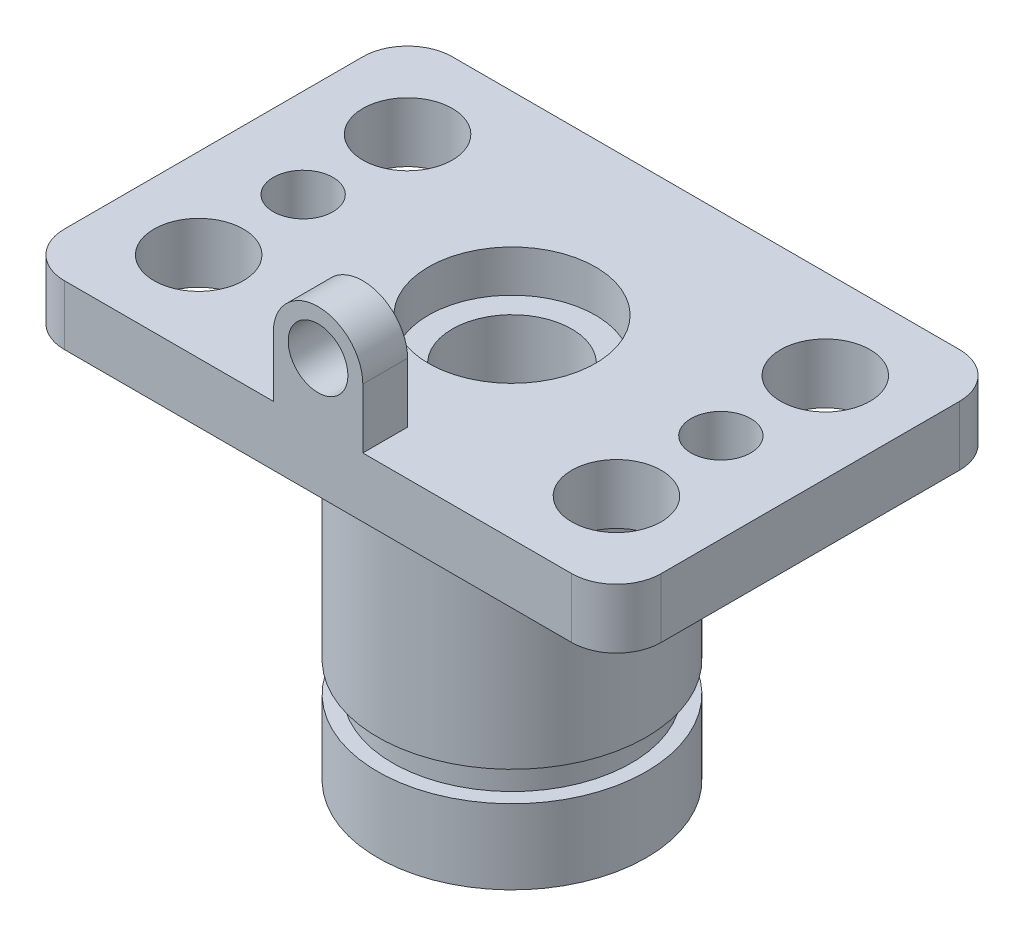
ISO-10303-21;
HEADER;
FILE_DESCRIPTION(('STEP AP214'),'2;1');
FILE_NAME('part.step','',(''),(''),'','','');
FILE_SCHEMA(('AUTOMOTIVE_DESIGN { 1 0 10303 214 1 1 1 1 }'));
ENDSEC;
DATA;
#1=APPLICATION_CONTEXT('core data for automotive mechanical design processes');
#2=APPLICATION_PROTOCOL_DEFINITION('international standard','automotive_design',2000,#1);
#3=PRODUCT_CONTEXT('',#1,'mechanical');
#4=PRODUCT('Part','Part','',(#3));
#5=PRODUCT_RELATED_PRODUCT_CATEGORY('part','',(#4));
#6=PRODUCT_DEFINITION_FORMATION('','',#4);
#7=PRODUCT_DEFINITION_CONTEXT('part definition',#1,'design');
#8=PRODUCT_DEFINITION('design','',#6,#7);
#9=PRODUCT_DEFINITION_SHAPE('','',#8);
#10=(LENGTH_UNIT() NAMED_UNIT(*) SI_UNIT(.MILLI.,.METRE.));
#11=(NAMED_UNIT(*) PLANE_ANGLE_UNIT() SI_UNIT($,.RADIAN.));
#12=(NAMED_UNIT(*) SI_UNIT($,.STERADIAN.) SOLID_ANGLE_UNIT());
#13=UNCERTAINTY_MEASURE_WITH_UNIT(LENGTH_MEASURE(1.E-05),#10,'distance_accuracy_value','');
#14=(GEOMETRIC_REPRESENTATION_CONTEXT(3) GLOBAL_UNCERTAINTY_ASSIGNED_CONTEXT((#13)) GLOBAL_UNIT_ASSIGNED_CONTEXT((#10,
#11,#12)) REPRESENTATION_CONTEXT('',''));
#15=CARTESIAN_POINT('',(0.,0.,0.));
#16=DIRECTION('',(0.,0.,1.));
#17=DIRECTION('',(1.,0.,0.));
#18=AXIS2_PLACEMENT_3D('',#15,#16,#17);
#19=CARTESIAN_POINT('',(0.,146.177983413139,0.));
#20=DIRECTION('',(0.,1.,0.));
#21=DIRECTION('',(-1.,0.,0.));
#22=AXIS2_PLACEMENT_3D('',#19,#20,#21);
#23=CYLINDRICAL_SURFACE('',#22,20.);
#24=CARTESIAN_POINT('',(0.,-57.5,0.));
#25=DIRECTION('',(0.,1.,0.));
#26=DIRECTION('',(-1.,0.,0.));
#27=AXIS2_PLACEMENT_3D('',#24,#25,#26);
#28=CIRCLE('',#27,20.);
#29=CARTESIAN_POINT('',(-20.,-57.5,0.));
#30=VERTEX_POINT('',#29);
#31=EDGE_CURVE('E48',#30,#30,#28,.T.);
#32=ORIENTED_EDGE('',*,*,#31,.F.);
#33=EDGE_LOOP('',(#32));
#34=FACE_BOUND('',#33,.T.);
#35=CARTESIAN_POINT('',(0.,63.5,0.));
#36=DIRECTION('',(0.,1.,0.));
#37=DIRECTION('',(-1.,0.,0.));
#38=AXIS2_PLACEMENT_3D('',#35,#36,#37);
#39=CIRCLE('',#38,20.);
#40=CARTESIAN_POINT('',(-20.,63.5,0.));
#41=VERTEX_POINT('',#40);
#42=EDGE_CURVE('E188',#41,#41,#39,.T.);
#43=ORIENTED_EDGE('',*,*,#42,.T.);
#44=EDGE_LOOP('',(#43));
#45=FACE_BOUND('',#44,.T.);
#46=ADVANCED_FACE('F41',(#34,#45),#23,.F.);
#47=CARTESIAN_POINT('',(-45.,-57.5,0.));
#48=DIRECTION('',(0.,-1.,0.));
#49=DIRECTION('',(1.,0.,0.));
#50=AXIS2_PLACEMENT_3D('',#47,#48,#49);
#51=PLANE('',#50);
#52=ORIENTED_EDGE('',*,*,#31,.T.);
#53=EDGE_LOOP('',(#52));
#54=FACE_BOUND('',#53,.T.);
#55=CARTESIAN_POINT('',(0.,-57.5,0.));
#56=DIRECTION('',(0.,1.,0.));
#57=DIRECTION('',(-1.,0.,0.));
#58=AXIS2_PLACEMENT_3D('',#55,#56,#57);
#59=CIRCLE('',#58,45.);
#60=CARTESIAN_POINT('',(-45.,-57.5,0.));
#61=VERTEX_POINT('',#60);
#62=EDGE_CURVE('E174',#61,#61,#59,.T.);
#63=ORIENTED_EDGE('',*,*,#62,.F.);
#64=EDGE_LOOP('',(#63));
#65=FACE_BOUND('',#64,.T.);
#66=ADVANCED_FACE('F178',(#54,#65),#51,.T.);
#67=CARTESIAN_POINT('',(0.,146.177983413139,0.));
#68=DIRECTION('',(0.,1.,0.));
#69=DIRECTION('',(-1.,0.,0.));
#70=AXIS2_PLACEMENT_3D('',#67,#68,#69);
#71=CYLINDRICAL_SURFACE('',#70,45.);
#72=ORIENTED_EDGE('',*,*,#62,.T.);
#73=EDGE_LOOP('',(#72));
#74=FACE_BOUND('',#73,.T.);
#75=CARTESIAN_POINT('',(0.,-32.5,0.));
#76=DIRECTION('',(0.,1.,0.));
#77=DIRECTION('',(-1.,0.,0.));
#78=AXIS2_PLACEMENT_3D('',#75,#76,#77);
#79=CIRCLE('',#78,45.);
#80=CARTESIAN_POINT('',(-45.,-32.5,0.));
#81=VERTEX_POINT('',#80);
#82=EDGE_CURVE('E173',#81,#81,#79,.T.);
#83=ORIENTED_EDGE('',*,*,#82,.F.);
#84=EDGE_LOOP('',(#83));
#85=FACE_BOUND('',#84,.T.);
#86=ADVANCED_FACE('F339',(#74,#85),#71,.T.);
#87=CARTESIAN_POINT('',(-45.,-32.5,0.));
#88=DIRECTION('',(0.,1.,0.));
#89=DIRECTION('',(-1.,0.,0.));
#90=AXIS2_PLACEMENT_3D('',#87,#88,#89);
#91=PLANE('',#90);
#92=ORIENTED_EDGE('',*,*,#82,.T.);
#93=EDGE_LOOP('',(#92));
#94=FACE_BOUND('',#93,.T.);
#95=CARTESIAN_POINT('',(0.,-32.5,0.));
#96=DIRECTION('',(0.,1.,0.));
#97=DIRECTION('',(-1.,0.,0.));
#98=AXIS2_PLACEMENT_3D('',#95,#96,#97);
#99=CIRCLE('',#98,40.);
#100=CARTESIAN_POINT('',(-40.,-32.5,0.));
#101=VERTEX_POINT('',#100);
#102=EDGE_CURVE('E169',#101,#101,#99,.T.);
#103=ORIENTED_EDGE('',*,*,#102,.F.);
#104=EDGE_LOOP('',(#103));
#105=FACE_BOUND('',#104,.T.);
#106=ADVANCED_FACE('F333',(#94,#105),#91,.T.);
#107=CARTESIAN_POINT('',(0.,146.177983413139,0.));
#108=DIRECTION('',(0.,1.,0.));
#109=DIRECTION('',(-1.,0.,0.));
#110=AXIS2_PLACEMENT_3D('',#107,#108,#109);
#111=CYLINDRICAL_SURFACE('',#110,40.);
#112=ORIENTED_EDGE('',*,*,#102,.T.);
#113=EDGE_LOOP('',(#112));
#114=FACE_BOUND('',#113,.T.);
#115=CARTESIAN_POINT('',(0.,-22.5,0.));
#116=DIRECTION('',(0.,1.,0.));
#117=DIRECTION('',(-1.,0.,0.));
#118=AXIS2_PLACEMENT_3D('',#115,#116,#117);
#119=CIRCLE('',#118,40.);
#120=CARTESIAN_POINT('',(-40.,-22.5,0.));
#121=VERTEX_POINT('',#120);
#122=EDGE_CURVE('E164',#121,#121,#119,.T.);
#123=ORIENTED_EDGE('',*,*,#122,.F.);
#124=EDGE_LOOP('',(#123));
#125=FACE_BOUND('',#124,.T.);
#126=ADVANCED_FACE('F326',(#114,#125),#111,.T.);
#127=CARTESIAN_POINT('',(-45.,-22.5,0.));
#128=DIRECTION('',(0.,-1.,0.));
#129=DIRECTION('',(1.,0.,0.));
#130=AXIS2_PLACEMENT_3D('',#127,#128,#129);
#131=PLANE('',#130);
#132=ORIENTED_EDGE('',*,*,#122,.T.);
#133=EDGE_LOOP('',(#132));
#134=FACE_BOUND('',#133,.T.);
#135=CARTESIAN_POINT('',(0.,-22.5,0.));
#136=DIRECTION('',(0.,1.,0.));
#137=DIRECTION('',(-1.,0.,0.));
#138=AXIS2_PLACEMENT_3D('',#135,#136,#137);
#139=CIRCLE('',#138,45.);
#140=CARTESIAN_POINT('',(-45.,-22.5,0.));
#141=VERTEX_POINT('',#140);
#142=EDGE_CURVE('E165',#141,#141,#139,.T.);
#143=ORIENTED_EDGE('',*,*,#142,.F.);
#144=EDGE_LOOP('',(#143));
#145=FACE_BOUND('',#144,.T.);
#146=ADVANCED_FACE('F319',(#134,#145),#131,.T.);
#147=CARTESIAN_POINT('',(0.,146.177983413139,0.));
#148=DIRECTION('',(0.,1.,0.));
#149=DIRECTION('',(-1.,0.,0.));
#150=AXIS2_PLACEMENT_3D('',#147,#148,#149);
#151=CYLINDRICAL_SURFACE('',#150,45.);
#152=ORIENTED_EDGE('',*,*,#142,.T.);
#153=EDGE_LOOP('',(#152));
#154=FACE_BOUND('',#153,.T.);
#155=CARTESIAN_POINT('',(0.,57.5,0.));
#156=DIRECTION('',(0.,1.,0.));
#157=DIRECTION('',(-1.,0.,0.));
#158=AXIS2_PLACEMENT_3D('',#155,#156,#157);
#159=CIRCLE('',#158,45.);
#160=CARTESIAN_POINT('',(-45.,57.5,0.));
#161=VERTEX_POINT('',#160);
#162=EDGE_CURVE('E157',#161,#161,#159,.T.);
#163=ORIENTED_EDGE('',*,*,#162,.F.);
#164=EDGE_LOOP('',(#163));
#165=FACE_BOUND('',#164,.T.);
#166=ADVANCED_FACE('F303',(#154,#165),#151,.T.);
#167=CARTESIAN_POINT('',(0.,57.5,0.));
#168=DIRECTION('',(0.,1.,0.));
#169=DIRECTION('',(-1.,0.,0.));
#170=AXIS2_PLACEMENT_3D('',#167,#168,#169);
#171=PLANE('',#170);
#172=CARTESIAN_POINT('',(70.,57.5,0.));
#173=DIRECTION('',(0.,1.,0.));
#174=DIRECTION('',(-1.,0.,0.));
#175=AXIS2_PLACEMENT_3D('',#172,#173,#174);
#176=CIRCLE('',#175,9.99999999999999);
#177=CARTESIAN_POINT('',(60.,57.5,0.));
#178=VERTEX_POINT('',#177);
#179=EDGE_CURVE('E226',#178,#178,#176,.F.);
#180=ORIENTED_EDGE('',*,*,#179,.F.);
#181=EDGE_LOOP('',(#180));
#182=FACE_BOUND('',#181,.T.);
#183=CARTESIAN_POINT('',(-70.,57.5,-35.));
#184=DIRECTION('',(0.,1.,0.));
#185=DIRECTION('',(-1.,0.,0.));
#186=AXIS2_PLACEMENT_3D('',#183,#184,#185);
#187=CIRCLE('',#186,15.);
#188=CARTESIAN_POINT('',(-85.,57.5,-35.));
#189=VERTEX_POINT('',#188);
#190=EDGE_CURVE('E295',#189,#189,#187,.F.);
#191=ORIENTED_EDGE('',*,*,#190,.F.);
#192=EDGE_LOOP('',(#191));
#193=FACE_BOUND('',#192,.T.);
#194=CARTESIAN_POINT('',(-70.,57.5,35.));
#195=DIRECTION('',(0.,1.,0.));
#196=DIRECTION('',(-1.,0.,0.));
#197=AXIS2_PLACEMENT_3D('',#194,#195,#196);
#198=CIRCLE('',#197,15.);
#199=CARTESIAN_POINT('',(-85.,57.5,35.));
#200=VERTEX_POINT('',#199);
#201=EDGE_CURVE('E288',#200,#200,#198,.T.);
#202=ORIENTED_EDGE('',*,*,#201,.T.);
#203=EDGE_LOOP('',(#202));
#204=FACE_BOUND('',#203,.T.);
#205=CARTESIAN_POINT('',(85.,57.5,-50.));
#206=DIRECTION('',(0.,1.,0.));
#207=DIRECTION('',(-1.,0.,0.));
#208=AXIS2_PLACEMENT_3D('',#205,#206,#207);
#209=CIRCLE('',#208,15.);
#210=CARTESIAN_POINT('',(85.,57.5,-65.));
#211=VERTEX_POINT('',#210);
#212=CARTESIAN_POINT('',(100.,57.5,-50.));
#213=VERTEX_POINT('',#212);
#214=EDGE_CURVE('E267',#211,#213,#209,.F.);
#215=ORIENTED_EDGE('',*,*,#214,.T.);
#216=DIRECTION('',(0.,0.,-1.));
#217=VECTOR('',#216,1.);
#218=CARTESIAN_POINT('',(100.,57.5,0.));
#219=LINE('',#218,#217);
#220=CARTESIAN_POINT('',(100.,57.5,50.));
#221=VERTEX_POINT('',#220);
#222=EDGE_CURVE('E287',#221,#213,#219,.T.);
#223=ORIENTED_EDGE('',*,*,#222,.F.);
#224=CARTESIAN_POINT('',(85.,57.5,50.));
#225=DIRECTION('',(0.,1.,0.));
#226=DIRECTION('',(-1.,0.,0.));
#227=AXIS2_PLACEMENT_3D('',#224,#225,#226);
#228=CIRCLE('',#227,15.);
#229=CARTESIAN_POINT('',(85.,57.5,65.));
#230=VERTEX_POINT('',#229);
#231=EDGE_CURVE('E282',#230,#221,#228,.T.);
#232=ORIENTED_EDGE('',*,*,#231,.F.);
#233=DIRECTION('',(1.,0.,0.));
#234=VECTOR('',#233,1.);
#235=CARTESIAN_POINT('',(0.,57.5,65.));
#236=LINE('',#235,#234);
#237=CARTESIAN_POINT('',(-85.,57.5,65.));
#238=VERTEX_POINT('',#237);
#239=EDGE_CURVE('E144',#238,#230,#236,.T.);
#240=ORIENTED_EDGE('',*,*,#239,.F.);
#241=CARTESIAN_POINT('',(-85.,57.5,50.));
#242=DIRECTION('',(0.,1.,0.));
#243=DIRECTION('',(-1.,0.,0.));
#244=AXIS2_PLACEMENT_3D('',#241,#242,#243);
#245=CIRCLE('',#244,15.);
#246=CARTESIAN_POINT('',(-100.,57.5,50.));
#247=VERTEX_POINT('',#246);
#248=EDGE_CURVE('E283',#238,#247,#245,.F.);
#249=ORIENTED_EDGE('',*,*,#248,.T.);
#250=DIRECTION('',(0.,0.,-1.));
#251=VECTOR('',#250,1.);
#252=CARTESIAN_POINT('',(-100.,57.5,0.));
#253=LINE('',#252,#251);
#254=CARTESIAN_POINT('',(-100.,57.5,-50.));
#255=VERTEX_POINT('',#254);
#256=EDGE_CURVE('E279',#247,#255,#253,.T.);
#257=ORIENTED_EDGE('',*,*,#256,.T.);
#258=CARTESIAN_POINT('',(-85.,57.5,-50.));
#259=DIRECTION('',(0.,1.,0.));
#260=DIRECTION('',(-1.,0.,0.));
#261=AXIS2_PLACEMENT_3D('',#258,#259,#260);
#262=CIRCLE('',#261,15.);
#263=CARTESIAN_POINT('',(-85.,57.5,-65.));
#264=VERTEX_POINT('',#263);
#265=EDGE_CURVE('E274',#255,#264,#262,.F.);
#266=ORIENTED_EDGE('',*,*,#265,.T.);
#267=DIRECTION('',(1.,0.,0.));
#268=VECTOR('',#267,1.);
#269=CARTESIAN_POINT('',(0.,57.5,-65.));
#270=LINE('',#269,#268);
#271=EDGE_CURVE('E275',#264,#211,#270,.T.);
#272=ORIENTED_EDGE('',*,*,#271,.T.);
#273=EDGE_LOOP('',(#215,#223,#232,#240,#249,#257,#266,#272));
#274=FACE_BOUND('',#273,.T.);
#275=CARTESIAN_POINT('',(-70.,57.5,0.));
#276=DIRECTION('',(0.,1.,0.));
#277=DIRECTION('',(-1.,0.,0.));
#278=AXIS2_PLACEMENT_3D('',#275,#276,#277);
#279=CIRCLE('',#278,10.);
#280=CARTESIAN_POINT('',(-80.,57.5,0.));
#281=VERTEX_POINT('',#280);
#282=EDGE_CURVE('E266',#281,#281,#279,.T.);
#283=ORIENTED_EDGE('',*,*,#282,.T.);
#284=EDGE_LOOP('',(#283));
#285=FACE_BOUND('',#284,.T.);
#286=CARTESIAN_POINT('',(70.,57.5,35.));
#287=DIRECTION('',(0.,1.,0.));
#288=DIRECTION('',(-1.,0.,0.));
#289=AXIS2_PLACEMENT_3D('',#286,#287,#288);
#290=CIRCLE('',#289,15.);
#291=CARTESIAN_POINT('',(55.,57.5,35.));
#292=VERTEX_POINT('',#291);
#293=EDGE_CURVE('E263',#292,#292,#290,.F.);
#294=ORIENTED_EDGE('',*,*,#293,.F.);
#295=EDGE_LOOP('',(#294));
#296=FACE_BOUND('',#295,.T.);
#297=CARTESIAN_POINT('',(70.,57.5,-35.));
#298=DIRECTION('',(0.,1.,0.));
#299=DIRECTION('',(-1.,0.,0.));
#300=AXIS2_PLACEMENT_3D('',#297,#298,#299);
#301=CIRCLE('',#300,15.);
#302=CARTESIAN_POINT('',(55.,57.5,-35.));
#303=VERTEX_POINT('',#302);
#304=EDGE_CURVE('E220',#303,#303,#301,.T.);
#305=ORIENTED_EDGE('',*,*,#304,.T.);
#306=EDGE_LOOP('',(#305));
#307=FACE_BOUND('',#306,.T.);
#308=ORIENTED_EDGE('',*,*,#162,.T.);
#309=EDGE_LOOP('',(#308));
#310=FACE_BOUND('',#309,.T.);
#311=ADVANCED_FACE('F297',(#182,#193,#204,#274,#285,#296,#307,#310),#171,.F.);
#312=CARTESIAN_POINT('',(85.,77.5,-50.));
#313=DIRECTION('',(0.,-1.,0.));
#314=DIRECTION('',(1.,0.,0.));
#315=AXIS2_PLACEMENT_3D('',#312,#313,#314);
#316=CYLINDRICAL_SURFACE('',#315,15.);
#317=ORIENTED_EDGE('',*,*,#214,.F.);
#318=DIRECTION('',(0.,-1.,0.));
#319=VECTOR('',#318,1.);
#320=CARTESIAN_POINT('',(85.,77.5,-65.));
#321=LINE('',#320,#319);
#322=CARTESIAN_POINT('',(85.,77.5,-65.));
#323=VERTEX_POINT('',#322);
#324=EDGE_CURVE('E105',#323,#211,#321,.T.);
#325=ORIENTED_EDGE('',*,*,#324,.F.);
#326=CARTESIAN_POINT('',(85.,77.5,-50.));
#327=DIRECTION('',(0.,1.,0.));
#328=DIRECTION('',(-1.,0.,0.));
#329=AXIS2_PLACEMENT_3D('',#326,#327,#328);
#330=CIRCLE('',#329,15.);
#331=CARTESIAN_POINT('',(100.,77.5,-50.));
#332=VERTEX_POINT('',#331);
#333=EDGE_CURVE('E233',#323,#332,#330,.F.);
#334=ORIENTED_EDGE('',*,*,#333,.T.);
#335=DIRECTION('',(0.,-1.,0.));
#336=VECTOR('',#335,1.);
#337=CARTESIAN_POINT('',(100.,77.5,-50.));
#338=LINE('',#337,#336);
#339=EDGE_CURVE('E100',#332,#213,#338,.T.);
#340=ORIENTED_EDGE('',*,*,#339,.T.);
#341=EDGE_LOOP('',(#317,#325,#334,#340));
#342=FACE_BOUND('',#341,.T.);
#343=ADVANCED_FACE('F304',(#342),#316,.T.);
#344=CARTESIAN_POINT('',(0.,77.5,-65.));
#345=DIRECTION('',(0.,0.,-1.));
#346=DIRECTION('',(-1.,0.,0.));
#347=AXIS2_PLACEMENT_3D('',#344,#345,#346);
#348=PLANE('',#347);
#349=ORIENTED_EDGE('',*,*,#271,.F.);
#350=DIRECTION('',(0.,-1.,0.));
#351=VECTOR('',#350,1.);
#352=CARTESIAN_POINT('',(-85.,77.5,-65.));
#353=LINE('',#352,#351);
#354=CARTESIAN_POINT('',(-85.,77.5,-65.));
#355=VERTEX_POINT('',#354);
#356=EDGE_CURVE('E156',#355,#264,#353,.T.);
#357=ORIENTED_EDGE('',*,*,#356,.F.);
#358=DIRECTION('',(1.,0.,0.));
#359=VECTOR('',#358,1.);
#360=CARTESIAN_POINT('',(0.,77.5,-65.));
#361=LINE('',#360,#359);
#362=EDGE_CURVE('E237',#355,#323,#361,.T.);
#363=ORIENTED_EDGE('',*,*,#362,.T.);
#364=ORIENTED_EDGE('',*,*,#324,.T.);
#365=EDGE_LOOP('',(#349,#357,#363,#364));
#366=FACE_BOUND('',#365,.T.);
#367=ADVANCED_FACE('F388',(#366),#348,.T.);
#368=CARTESIAN_POINT('',(-85.,77.5,-50.));
#369=DIRECTION('',(0.,-1.,0.));
#370=DIRECTION('',(1.,0.,0.));
#371=AXIS2_PLACEMENT_3D('',#368,#369,#370);
#372=CYLINDRICAL_SURFACE('',#371,15.);
#373=ORIENTED_EDGE('',*,*,#265,.F.);
#374=DIRECTION('',(0.,-1.,0.));
#375=VECTOR('',#374,1.);
#376=CARTESIAN_POINT('',(-100.,77.5,-50.));
#377=LINE('',#376,#375);
#378=CARTESIAN_POINT('',(-100.,77.5,-50.));
#379=VERTEX_POINT('',#378);
#380=EDGE_CURVE('E152',#379,#255,#377,.T.);
#381=ORIENTED_EDGE('',*,*,#380,.F.);
#382=CARTESIAN_POINT('',(-85.,77.5,-50.));
#383=DIRECTION('',(0.,1.,0.));
#384=DIRECTION('',(-1.,0.,0.));
#385=AXIS2_PLACEMENT_3D('',#382,#383,#384);
#386=CIRCLE('',#385,15.);
#387=EDGE_CURVE('E239',#379,#355,#386,.F.);
#388=ORIENTED_EDGE('',*,*,#387,.T.);
#389=ORIENTED_EDGE('',*,*,#356,.T.);
#390=EDGE_LOOP('',(#373,#381,#388,#389));
#391=FACE_BOUND('',#390,.T.);
#392=ADVANCED_FACE('F398',(#391),#372,.T.);
#393=CARTESIAN_POINT('',(-100.,77.5,0.));
#394=DIRECTION('',(-1.,0.,0.));
#395=DIRECTION('',(0.,-1.,0.));
#396=AXIS2_PLACEMENT_3D('',#393,#394,#395);
#397=PLANE('',#396);
#398=ORIENTED_EDGE('',*,*,#256,.F.);
#399=DIRECTION('',(0.,-1.,0.));
#400=VECTOR('',#399,1.);
#401=CARTESIAN_POINT('',(-100.,77.5,50.));
#402=LINE('',#401,#400);
#403=CARTESIAN_POINT('',(-100.,77.5,50.));
#404=VERTEX_POINT('',#403);
#405=EDGE_CURVE('E146',#404,#247,#402,.T.);
#406=ORIENTED_EDGE('',*,*,#405,.F.);
#407=DIRECTION('',(0.,0.,-1.));
#408=VECTOR('',#407,1.);
#409=CARTESIAN_POINT('',(-100.,77.5,0.));
#410=LINE('',#409,#408);
#411=EDGE_CURVE('E245',#404,#379,#410,.T.);
#412=ORIENTED_EDGE('',*,*,#411,.T.);
#413=ORIENTED_EDGE('',*,*,#380,.T.);
#414=EDGE_LOOP('',(#398,#406,#412,#413));
#415=FACE_BOUND('',#414,.T.);
#416=ADVANCED_FACE('F409',(#415),#397,.T.);
#417=CARTESIAN_POINT('',(-85.,77.5,50.));
#418=DIRECTION('',(0.,-1.,0.));
#419=DIRECTION('',(1.,0.,0.));
#420=AXIS2_PLACEMENT_3D('',#417,#418,#419);
#421=CYLINDRICAL_SURFACE('',#420,15.);
#422=ORIENTED_EDGE('',*,*,#248,.F.);
#423=DIRECTION('',(0.,-1.,0.));
#424=VECTOR('',#423,1.);
#425=CARTESIAN_POINT('',(-85.,77.5,65.));
#426=LINE('',#425,#424);
#427=CARTESIAN_POINT('',(-85.,77.5,65.));
#428=VERTEX_POINT('',#427);
#429=EDGE_CURVE('E148',#428,#238,#426,.T.);
#430=ORIENTED_EDGE('',*,*,#429,.F.);
#431=CARTESIAN_POINT('',(-85.,77.5,50.));
#432=DIRECTION('',(0.,1.,0.));
#433=DIRECTION('',(-1.,0.,0.));
#434=AXIS2_PLACEMENT_3D('',#431,#432,#433);
#435=CIRCLE('',#434,15.);
#436=EDGE_CURVE('E133',#428,#404,#435,.F.);
#437=ORIENTED_EDGE('',*,*,#436,.T.);
#438=ORIENTED_EDGE('',*,*,#405,.T.);
#439=EDGE_LOOP('',(#422,#430,#437,#438));
#440=FACE_BOUND('',#439,.T.);
#441=ADVANCED_FACE('F420',(#440),#421,.T.);
#442=CARTESIAN_POINT('',(0.,77.5,65.));
#443=DIRECTION('',(0.,0.,-1.));
#444=DIRECTION('',(-1.,0.,0.));
#445=AXIS2_PLACEMENT_3D('',#442,#443,#444);
#446=PLANE('',#445);
#447=ORIENTED_EDGE('',*,*,#239,.T.);
#448=DIRECTION('',(0.,-1.,0.));
#449=VECTOR('',#448,1.);
#450=CARTESIAN_POINT('',(85.,77.5,65.));
#451=LINE('',#450,#449);
#452=CARTESIAN_POINT('',(85.,77.5,65.));
#453=VERTEX_POINT('',#452);
#454=EDGE_CURVE('E137',#453,#230,#451,.T.);
#455=ORIENTED_EDGE('',*,*,#454,.F.);
#456=DIRECTION('',(1.,0.,0.));
#457=VECTOR('',#456,1.);
#458=CARTESIAN_POINT('',(0.,77.5,65.));
#459=LINE('',#458,#457);
#460=CARTESIAN_POINT('',(15.,77.5,65.));
#461=VERTEX_POINT('',#460);
#462=EDGE_CURVE('E119',#461,#453,#459,.T.);
#463=ORIENTED_EDGE('',*,*,#462,.F.);
#464=DIRECTION('',(0.,1.,0.));
#465=VECTOR('',#464,1.);
#466=CARTESIAN_POINT('',(15.,97.5,65.));
#467=LINE('',#466,#465);
#468=CARTESIAN_POINT('',(15.,97.5,65.));
#469=VERTEX_POINT('',#468);
#470=EDGE_CURVE('E54',#461,#469,#467,.T.);
#471=ORIENTED_EDGE('',*,*,#470,.T.);
#472=CARTESIAN_POINT('',(0.,97.5,65.));
#473=DIRECTION('',(0.,0.,1.));
#474=DIRECTION('',(1.,0.,0.));
#475=AXIS2_PLACEMENT_3D('',#472,#473,#474);
#476=CIRCLE('',#475,15.);
#477=CARTESIAN_POINT('',(-15.,97.5,65.));
#478=VERTEX_POINT('',#477);
#479=EDGE_CURVE('E195',#469,#478,#476,.T.);
#480=ORIENTED_EDGE('',*,*,#479,.T.);
#481=DIRECTION('',(0.,-1.,0.));
#482=VECTOR('',#481,1.);
#483=CARTESIAN_POINT('',(-15.,97.5,65.));
#484=LINE('',#483,#482);
#485=CARTESIAN_POINT('',(-15.,77.5,65.));
#486=VERTEX_POINT('',#485);
#487=EDGE_CURVE('E211',#478,#486,#484,.T.);
#488=ORIENTED_EDGE('',*,*,#487,.T.);
#489=EDGE_CURVE('E128',#428,#486,#459,.T.);
#490=ORIENTED_EDGE('',*,*,#489,.F.);
#491=ORIENTED_EDGE('',*,*,#429,.T.);
#492=EDGE_LOOP('',(#447,#455,#463,#471,#480,#488,#490,#491));
#493=FACE_BOUND('',#492,.T.);
#494=CARTESIAN_POINT('',(0.,97.5,65.));
#495=DIRECTION('',(0.,0.,1.));
#496=DIRECTION('',(1.,0.,0.));
#497=AXIS2_PLACEMENT_3D('',#494,#495,#496);
#498=CIRCLE('',#497,10.);
#499=CARTESIAN_POINT('',(10.,97.5,65.));
#500=VERTEX_POINT('',#499);
#501=EDGE_CURVE('E186',#500,#500,#498,.T.);
#502=ORIENTED_EDGE('',*,*,#501,.F.);
#503=EDGE_LOOP('',(#502));
#504=FACE_BOUND('',#503,.T.);
#505=ADVANCED_FACE('F142',(#493,#504),#446,.F.);
#506=CARTESIAN_POINT('',(85.,77.5,50.));
#507=DIRECTION('',(0.,-1.,0.));
#508=DIRECTION('',(1.,0.,0.));
#509=AXIS2_PLACEMENT_3D('',#506,#507,#508);
#510=CYLINDRICAL_SURFACE('',#509,15.);
#511=ORIENTED_EDGE('',*,*,#231,.T.);
#512=DIRECTION('',(0.,-1.,0.));
#513=VECTOR('',#512,1.);
#514=CARTESIAN_POINT('',(100.,77.5,50.));
#515=LINE('',#514,#513);
#516=CARTESIAN_POINT('',(100.,77.5,50.));
#517=VERTEX_POINT('',#516);
#518=EDGE_CURVE('E140',#517,#221,#515,.T.);
#519=ORIENTED_EDGE('',*,*,#518,.F.);
#520=CARTESIAN_POINT('',(85.,77.5,50.));
#521=DIRECTION('',(0.,1.,0.));
#522=DIRECTION('',(-1.,0.,0.));
#523=AXIS2_PLACEMENT_3D('',#520,#521,#522);
#524=CIRCLE('',#523,15.);
#525=EDGE_CURVE('E123',#453,#517,#524,.T.);
#526=ORIENTED_EDGE('',*,*,#525,.F.);
#527=ORIENTED_EDGE('',*,*,#454,.T.);
#528=EDGE_LOOP('',(#511,#519,#526,#527));
#529=FACE_BOUND('',#528,.T.);
#530=ADVANCED_FACE('F136',(#529),#510,.T.);
#531=CARTESIAN_POINT('',(70.,77.5,0.));
#532=DIRECTION('',(0.,-1.,0.));
#533=DIRECTION('',(1.,0.,0.));
#534=AXIS2_PLACEMENT_3D('',#531,#532,#533);
#535=CYLINDRICAL_SURFACE('',#534,9.99999999999999);
#536=CARTESIAN_POINT('',(70.,77.5,0.));
#537=DIRECTION('',(0.,1.,0.));
#538=DIRECTION('',(-1.,0.,0.));
#539=AXIS2_PLACEMENT_3D('',#536,#537,#538);
#540=CIRCLE('',#539,9.99999999999999);
#541=CARTESIAN_POINT('',(60.,77.5,0.));
#542=VERTEX_POINT('',#541);
#543=EDGE_CURVE('E254',#542,#542,#540,.F.);
#544=ORIENTED_EDGE('',*,*,#543,.F.);
#545=EDGE_LOOP('',(#544));
#546=FACE_BOUND('',#545,.T.);
#547=ORIENTED_EDGE('',*,*,#179,.T.);
#548=EDGE_LOOP('',(#547));
#549=FACE_BOUND('',#548,.T.);
#550=ADVANCED_FACE('F296',(#546,#549),#535,.F.);
#551=CARTESIAN_POINT('',(-70.,77.5,-35.));
#552=DIRECTION('',(0.,-1.,0.));
#553=DIRECTION('',(1.,0.,0.));
#554=AXIS2_PLACEMENT_3D('',#551,#552,#553);
#555=CYLINDRICAL_SURFACE('',#554,15.);
#556=CARTESIAN_POINT('',(-70.,77.5,-35.));
#557=DIRECTION('',(0.,1.,0.));
#558=DIRECTION('',(-1.,0.,0.));
#559=AXIS2_PLACEMENT_3D('',#556,#557,#558);
#560=CIRCLE('',#559,15.);
#561=CARTESIAN_POINT('',(-85.,77.5,-35.));
#562=VERTEX_POINT('',#561);
#563=EDGE_CURVE('E252',#562,#562,#560,.F.);
#564=ORIENTED_EDGE('',*,*,#563,.F.);
#565=EDGE_LOOP('',(#564));
#566=FACE_BOUND('',#565,.T.);
#567=ORIENTED_EDGE('',*,*,#190,.T.);
#568=EDGE_LOOP('',(#567));
#569=FACE_BOUND('',#568,.T.);
#570=ADVANCED_FACE('F456',(#566,#569),#555,.F.);
#571=CARTESIAN_POINT('',(-70.,77.5,35.));
#572=DIRECTION('',(0.,-1.,0.));
#573=DIRECTION('',(1.,0.,0.));
#574=AXIS2_PLACEMENT_3D('',#571,#572,#573);
#575=CYLINDRICAL_SURFACE('',#574,15.);
#576=CARTESIAN_POINT('',(-70.,77.5,35.));
#577=DIRECTION('',(0.,1.,0.));
#578=DIRECTION('',(-1.,0.,0.));
#579=AXIS2_PLACEMENT_3D('',#576,#577,#578);
#580=CIRCLE('',#579,15.);
#581=CARTESIAN_POINT('',(-85.,77.5,35.));
#582=VERTEX_POINT('',#581);
#583=EDGE_CURVE('E248',#582,#582,#580,.T.);
#584=ORIENTED_EDGE('',*,*,#583,.T.);
#585=EDGE_LOOP('',(#584));
#586=FACE_BOUND('',#585,.T.);
#587=ORIENTED_EDGE('',*,*,#201,.F.);
#588=EDGE_LOOP('',(#587));
#589=FACE_BOUND('',#588,.T.);
#590=ADVANCED_FACE('F469',(#586,#589),#575,.F.);
#591=CARTESIAN_POINT('',(100.,77.5,0.));
#592=DIRECTION('',(-1.,0.,0.));
#593=DIRECTION('',(0.,-1.,0.));
#594=AXIS2_PLACEMENT_3D('',#591,#592,#593);
#595=PLANE('',#594);
#596=ORIENTED_EDGE('',*,*,#222,.T.);
#597=ORIENTED_EDGE('',*,*,#339,.F.);
#598=DIRECTION('',(0.,0.,-1.));
#599=VECTOR('',#598,1.);
#600=CARTESIAN_POINT('',(100.,77.5,0.));
#601=LINE('',#600,#599);
#602=EDGE_CURVE('E64',#517,#332,#601,.T.);
#603=ORIENTED_EDGE('',*,*,#602,.F.);
#604=ORIENTED_EDGE('',*,*,#518,.T.);
#605=EDGE_LOOP('',(#596,#597,#603,#604));
#606=FACE_BOUND('',#605,.T.);
#607=ADVANCED_FACE('F476',(#606),#595,.F.);
#608=CARTESIAN_POINT('',(-70.,77.5,0.));
#609=DIRECTION('',(0.,-1.,0.));
#610=DIRECTION('',(1.,0.,0.));
#611=AXIS2_PLACEMENT_3D('',#608,#609,#610);
#612=CYLINDRICAL_SURFACE('',#611,10.);
#613=CARTESIAN_POINT('',(-70.,77.5,0.));
#614=DIRECTION('',(0.,1.,0.));
#615=DIRECTION('',(-1.,0.,0.));
#616=AXIS2_PLACEMENT_3D('',#613,#614,#615);
#617=CIRCLE('',#616,10.);
#618=CARTESIAN_POINT('',(-80.,77.5,0.));
#619=VERTEX_POINT('',#618);
#620=EDGE_CURVE('E231',#619,#619,#617,.T.);
#621=ORIENTED_EDGE('',*,*,#620,.T.);
#622=EDGE_LOOP('',(#621));
#623=FACE_BOUND('',#622,.T.);
#624=ORIENTED_EDGE('',*,*,#282,.F.);
#625=EDGE_LOOP('',(#624));
#626=FACE_BOUND('',#625,.T.);
#627=ADVANCED_FACE('F488',(#623,#626),#612,.F.);
#628=CARTESIAN_POINT('',(70.,77.5,35.));
#629=DIRECTION('',(0.,-1.,0.));
#630=DIRECTION('',(1.,0.,0.));
#631=AXIS2_PLACEMENT_3D('',#628,#629,#630);
#632=CYLINDRICAL_SURFACE('',#631,15.);
#633=CARTESIAN_POINT('',(70.,77.5,35.));
#634=DIRECTION('',(0.,1.,0.));
#635=DIRECTION('',(-1.,0.,0.));
#636=AXIS2_PLACEMENT_3D('',#633,#634,#635);
#637=CIRCLE('',#636,15.);
#638=CARTESIAN_POINT('',(55.,77.5,35.));
#639=VERTEX_POINT('',#638);
#640=EDGE_CURVE('E230',#639,#639,#637,.F.);
#641=ORIENTED_EDGE('',*,*,#640,.F.);
#642=EDGE_LOOP('',(#641));
#643=FACE_BOUND('',#642,.T.);
#644=ORIENTED_EDGE('',*,*,#293,.T.);
#645=EDGE_LOOP('',(#644));
#646=FACE_BOUND('',#645,.T.);
#647=ADVANCED_FACE('F499',(#643,#646),#632,.F.);
#648=CARTESIAN_POINT('',(70.,77.5,-35.));
#649=DIRECTION('',(0.,-1.,0.));
#650=DIRECTION('',(1.,0.,0.));
#651=AXIS2_PLACEMENT_3D('',#648,#649,#650);
#652=CYLINDRICAL_SURFACE('',#651,15.);
#653=CARTESIAN_POINT('',(70.,77.5,-35.));
#654=DIRECTION('',(0.,1.,0.));
#655=DIRECTION('',(-1.,0.,0.));
#656=AXIS2_PLACEMENT_3D('',#653,#654,#655);
#657=CIRCLE('',#656,15.);
#658=CARTESIAN_POINT('',(55.,77.5,-35.));
#659=VERTEX_POINT('',#658);
#660=EDGE_CURVE('E221',#659,#659,#657,.T.);
#661=ORIENTED_EDGE('',*,*,#660,.T.);
#662=EDGE_LOOP('',(#661));
#663=FACE_BOUND('',#662,.T.);
#664=ORIENTED_EDGE('',*,*,#304,.F.);
#665=EDGE_LOOP('',(#664));
#666=FACE_BOUND('',#665,.T.);
#667=ADVANCED_FACE('F329',(#663,#666),#652,.F.);
#668=CARTESIAN_POINT('',(0.,77.5,0.));
#669=DIRECTION('',(0.,-1.,0.));
#670=DIRECTION('',(1.,0.,0.));
#671=AXIS2_PLACEMENT_3D('',#668,#669,#670);
#672=CYLINDRICAL_SURFACE('',#671,28.);
#673=CARTESIAN_POINT('',(0.,63.5,0.));
#674=DIRECTION('',(0.,1.,0.));
#675=DIRECTION('',(-1.,0.,0.));
#676=AXIS2_PLACEMENT_3D('',#673,#674,#675);
#677=CIRCLE('',#676,28.);
#678=CARTESIAN_POINT('',(-28.,63.5,0.));
#679=VERTEX_POINT('',#678);
#680=EDGE_CURVE('E11',#679,#679,#677,.T.);
#681=ORIENTED_EDGE('',*,*,#680,.F.);
#682=EDGE_LOOP('',(#681));
#683=FACE_BOUND('',#682,.T.);
#684=CARTESIAN_POINT('',(0.,77.5,0.));
#685=DIRECTION('',(0.,1.,0.));
#686=DIRECTION('',(-1.,0.,0.));
#687=AXIS2_PLACEMENT_3D('',#684,#685,#686);
#688=CIRCLE('',#687,28.);
#689=CARTESIAN_POINT('',(-28.,77.5,0.));
#690=VERTEX_POINT('',#689);
#691=EDGE_CURVE('E256',#690,#690,#688,.T.);
#692=ORIENTED_EDGE('',*,*,#691,.T.);
#693=EDGE_LOOP('',(#692));
#694=FACE_BOUND('',#693,.T.);
#695=ADVANCED_FACE('F518',(#683,#694),#672,.F.);
#696=CARTESIAN_POINT('',(0.,77.5,0.));
#697=DIRECTION('',(0.,1.,0.));
#698=DIRECTION('',(-1.,0.,0.));
#699=AXIS2_PLACEMENT_3D('',#696,#697,#698);
#700=PLANE('',#699);
#701=DIRECTION('',(0.,0.,1.));
#702=VECTOR('',#701,1.);
#703=CARTESIAN_POINT('',(-15.,77.5,50.));
#704=LINE('',#703,#702);
#705=CARTESIAN_POINT('',(-15.,77.5,50.));
#706=VERTEX_POINT('',#705);
#707=EDGE_CURVE('E218',#706,#486,#704,.T.);
#708=ORIENTED_EDGE('',*,*,#707,.F.);
#709=DIRECTION('',(1.,0.,0.));
#710=VECTOR('',#709,1.);
#711=CARTESIAN_POINT('',(-15.,77.5,50.));
#712=LINE('',#711,#710);
#713=CARTESIAN_POINT('',(15.,77.5,50.));
#714=VERTEX_POINT('',#713);
#715=EDGE_CURVE('E201',#706,#714,#712,.T.);
#716=ORIENTED_EDGE('',*,*,#715,.T.);
#717=DIRECTION('',(0.,0.,1.));
#718=VECTOR('',#717,1.);
#719=CARTESIAN_POINT('',(15.,77.5,50.));
#720=LINE('',#719,#718);
#721=EDGE_CURVE('E130',#714,#461,#720,.T.);
#722=ORIENTED_EDGE('',*,*,#721,.T.);
#723=ORIENTED_EDGE('',*,*,#462,.T.);
#724=ORIENTED_EDGE('',*,*,#525,.T.);
#725=ORIENTED_EDGE('',*,*,#602,.T.);
#726=ORIENTED_EDGE('',*,*,#333,.F.);
#727=ORIENTED_EDGE('',*,*,#362,.F.);
#728=ORIENTED_EDGE('',*,*,#387,.F.);
#729=ORIENTED_EDGE('',*,*,#411,.F.);
#730=ORIENTED_EDGE('',*,*,#436,.F.);
#731=ORIENTED_EDGE('',*,*,#489,.T.);
#732=EDGE_LOOP('',(#708,#716,#722,#723,#724,#725,#726,#727,#728,#729,#730,#731));
#733=FACE_BOUND('',#732,.T.);
#734=ORIENTED_EDGE('',*,*,#660,.F.);
#735=EDGE_LOOP('',(#734));
#736=FACE_BOUND('',#735,.T.);
#737=ORIENTED_EDGE('',*,*,#640,.T.);
#738=EDGE_LOOP('',(#737));
#739=FACE_BOUND('',#738,.T.);
#740=ORIENTED_EDGE('',*,*,#620,.F.);
#741=EDGE_LOOP('',(#740));
#742=FACE_BOUND('',#741,.T.);
#743=ORIENTED_EDGE('',*,*,#583,.F.);
#744=EDGE_LOOP('',(#743));
#745=FACE_BOUND('',#744,.T.);
#746=ORIENTED_EDGE('',*,*,#563,.T.);
#747=EDGE_LOOP('',(#746));
#748=FACE_BOUND('',#747,.T.);
#749=ORIENTED_EDGE('',*,*,#543,.T.);
#750=EDGE_LOOP('',(#749));
#751=FACE_BOUND('',#750,.T.);
#752=ORIENTED_EDGE('',*,*,#691,.F.);
#753=EDGE_LOOP('',(#752));
#754=FACE_BOUND('',#753,.T.);
#755=ADVANCED_FACE('F122',(#733,#736,#739,#742,#745,#748,#751,#754),#700,.T.);
#756=CARTESIAN_POINT('',(0.,97.5,50.));
#757=DIRECTION('',(0.,0.,1.));
#758=DIRECTION('',(1.,0.,0.));
#759=AXIS2_PLACEMENT_3D('',#756,#757,#758);
#760=CYLINDRICAL_SURFACE('',#759,15.);
#761=ORIENTED_EDGE('',*,*,#479,.F.);
#762=DIRECTION('',(0.,0.,1.));
#763=VECTOR('',#762,1.);
#764=CARTESIAN_POINT('',(15.,97.5,50.));
#765=LINE('',#764,#763);
#766=CARTESIAN_POINT('',(15.,97.5,50.));
#767=VERTEX_POINT('',#766);
#768=EDGE_CURVE('E214',#767,#469,#765,.T.);
#769=ORIENTED_EDGE('',*,*,#768,.F.);
#770=CARTESIAN_POINT('',(0.,97.5,50.));
#771=DIRECTION('',(0.,0.,1.));
#772=DIRECTION('',(1.,0.,0.));
#773=AXIS2_PLACEMENT_3D('',#770,#771,#772);
#774=CIRCLE('',#773,15.);
#775=CARTESIAN_POINT('',(-15.,97.5,50.));
#776=VERTEX_POINT('',#775);
#777=EDGE_CURVE('E197',#767,#776,#774,.T.);
#778=ORIENTED_EDGE('',*,*,#777,.T.);
#779=DIRECTION('',(0.,0.,1.));
#780=VECTOR('',#779,1.);
#781=CARTESIAN_POINT('',(-15.,97.5,50.));
#782=LINE('',#781,#780);
#783=EDGE_CURVE('E208',#776,#478,#782,.T.);
#784=ORIENTED_EDGE('',*,*,#783,.T.);
#785=EDGE_LOOP('',(#761,#769,#778,#784));
#786=FACE_BOUND('',#785,.T.);
#787=ADVANCED_FACE('F534',(#786),#760,.T.);
#788=CARTESIAN_POINT('',(15.,97.5,50.));
#789=DIRECTION('',(1.,0.,0.));
#790=DIRECTION('',(0.,1.,0.));
#791=AXIS2_PLACEMENT_3D('',#788,#789,#790);
#792=PLANE('',#791);
#793=ORIENTED_EDGE('',*,*,#470,.F.);
#794=ORIENTED_EDGE('',*,*,#721,.F.);
#795=DIRECTION('',(0.,1.,0.));
#796=VECTOR('',#795,1.);
#797=CARTESIAN_POINT('',(15.,97.5,50.));
#798=LINE('',#797,#796);
#799=EDGE_CURVE('E202',#714,#767,#798,.T.);
#800=ORIENTED_EDGE('',*,*,#799,.T.);
#801=ORIENTED_EDGE('',*,*,#768,.T.);
#802=EDGE_LOOP('',(#793,#794,#800,#801));
#803=FACE_BOUND('',#802,.T.);
#804=ADVANCED_FACE('F546',(#803),#792,.T.);
#805=CARTESIAN_POINT('',(-15.,97.5,50.));
#806=DIRECTION('',(-1.,0.,0.));
#807=DIRECTION('',(0.,-1.,0.));
#808=AXIS2_PLACEMENT_3D('',#805,#806,#807);
#809=PLANE('',#808);
#810=ORIENTED_EDGE('',*,*,#487,.F.);
#811=ORIENTED_EDGE('',*,*,#783,.F.);
#812=DIRECTION('',(0.,-1.,0.));
#813=VECTOR('',#812,1.);
#814=CARTESIAN_POINT('',(-15.,97.5,50.));
#815=LINE('',#814,#813);
#816=EDGE_CURVE('E199',#776,#706,#815,.T.);
#817=ORIENTED_EDGE('',*,*,#816,.T.);
#818=ORIENTED_EDGE('',*,*,#707,.T.);
#819=EDGE_LOOP('',(#810,#811,#817,#818));
#820=FACE_BOUND('',#819,.T.);
#821=ADVANCED_FACE('F551',(#820),#809,.T.);
#822=CARTESIAN_POINT('',(0.,97.5,50.));
#823=DIRECTION('',(0.,0.,1.));
#824=DIRECTION('',(1.,0.,0.));
#825=AXIS2_PLACEMENT_3D('',#822,#823,#824);
#826=PLANE('',#825);
#827=CARTESIAN_POINT('',(0.,97.5,50.));
#828=DIRECTION('',(0.,0.,1.));
#829=DIRECTION('',(1.,0.,0.));
#830=AXIS2_PLACEMENT_3D('',#827,#828,#829);
#831=CIRCLE('',#830,10.);
#832=CARTESIAN_POINT('',(10.,97.5,50.));
#833=VERTEX_POINT('',#832);
#834=EDGE_CURVE('E191',#833,#833,#831,.T.);
#835=ORIENTED_EDGE('',*,*,#834,.T.);
#836=EDGE_LOOP('',(#835));
#837=FACE_BOUND('',#836,.T.);
#838=ORIENTED_EDGE('',*,*,#777,.F.);
#839=ORIENTED_EDGE('',*,*,#799,.F.);
#840=ORIENTED_EDGE('',*,*,#715,.F.);
#841=ORIENTED_EDGE('',*,*,#816,.F.);
#842=EDGE_LOOP('',(#838,#839,#840,#841));
#843=FACE_BOUND('',#842,.T.);
#844=ADVANCED_FACE('F562',(#837,#843),#826,.F.);
#845=CARTESIAN_POINT('',(0.,97.5,50.));
#846=DIRECTION('',(0.,0.,1.));
#847=DIRECTION('',(1.,0.,0.));
#848=AXIS2_PLACEMENT_3D('',#845,#846,#847);
#849=CYLINDRICAL_SURFACE('',#848,10.);
#850=ORIENTED_EDGE('',*,*,#834,.F.);
#851=EDGE_LOOP('',(#850));
#852=FACE_BOUND('',#851,.T.);
#853=ORIENTED_EDGE('',*,*,#501,.T.);
#854=EDGE_LOOP('',(#853));
#855=FACE_BOUND('',#854,.T.);
#856=ADVANCED_FACE('F575',(#852,#855),#849,.F.);
#857=CARTESIAN_POINT('',(0.,63.5,0.));
#858=DIRECTION('',(0.,1.,0.));
#859=DIRECTION('',(-1.,0.,0.));
#860=AXIS2_PLACEMENT_3D('',#857,#858,#859);
#861=PLANE('',#860);
#862=ORIENTED_EDGE('',*,*,#680,.T.);
#863=EDGE_LOOP('',(#862));
#864=FACE_BOUND('',#863,.T.);
#865=ORIENTED_EDGE('',*,*,#42,.F.);
#866=EDGE_LOOP('',(#865));
#867=FACE_BOUND('',#866,.T.);
#868=ADVANCED_FACE('F578',(#864,#867),#861,.T.);
#869=CLOSED_SHELL('',(#46,#66,#86,#106,#126,#146,#166,#311,#343,#367,#392,#416,#441,#505,#530,
#550,#570,#590,#607,#627,#647,#667,#695,#755,#787,#804,#821,#844,#856,#868));
#870=MANIFOLD_SOLID_BREP('B2',#869);
#871=ADVANCED_BREP_SHAPE_REPRESENTATION('',(#18,#870),#14);
#872=SHAPE_DEFINITION_REPRESENTATION(#9,#871);
ENDSEC;
END-ISO-10303-21;
